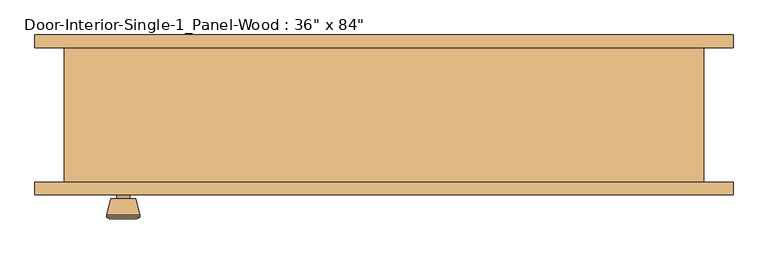
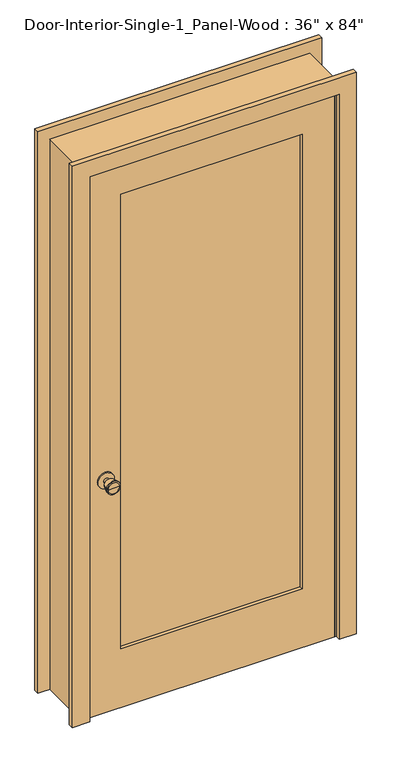
"""IFC4 building model written with IfcOpenShell, lengths in millimetres: door geometry."""

from ifc_helpers import new_model, si_unit, point, frame, frame_2d, origin, place, context, project, spatial, polyline, circle_curve, trimmed, segment, composite_curve, outline, extrude, faceted_brep, source, transform, mapped, element, save
from ifc_brep_helpers import plane_surface, cylinder_surface, revolved_surface, advanced_brep


def door_1a936fe1(model_context):
    return source(origin(), model_context, "Body", "SolidModel", [
        advanced_brep(
        [(-393.7, -57.5, 914.4), (-403.7, -57.5, 914.4), (-383.7, -57.5, 914.4), (-373.2241324, -8.5, 914.4), (-414.1758676, -8.5, 914.4), (-393.7, -8.5, 914.4), (-368.7, -10.3278681, 914.4), (-418.7, -10.3278681, 914.4), (-368.7, -13.7915463, 914.4), (-418.7, -13.7915463, 914.4), (-375.063764, -38.5, 914.4), (-412.336236, -38.5, 914.4), (-383.7, -38.5, 914.4), (-403.7, -38.5, 914.4)],
        [
            (0, 1),
            (1, 2, circle_curve(frame((-393.7, -57.5, 914.4), z_axis=(0.0, -1.0, 0.0), x_axis=(-1.0, 0.0, 0.0)), 10.0)),
            (2, 0),
            (2, 1, circle_curve(frame((-393.7, -57.5, 914.4), z_axis=(0.0, -1.0, 0.0), x_axis=(-1.0, 0.0, 0.0)), 10.0)),
            (3, 4, circle_curve(frame((-393.7, -8.5, 914.4), z_axis=(0.0, 1.0, 0.0), x_axis=(-1.0, 0.0, 0.0)), 20.4758676)),
            (4, 5),
            (5, 3),
            (4, 3, circle_curve(frame((-393.7, -8.5, 914.4), z_axis=(0.0, 1.0, 0.0), x_axis=(-1.0, 0.0, 0.0)), 20.4758676)),
            (6, 7, circle_curve(frame((-393.7, -10.3278681, 914.4), z_axis=(0.0, 1.0, 0.0), x_axis=(-1.0, 0.0, 0.0)), 25.0)),
            (7, 4),
            (3, 6),
            (7, 6, circle_curve(frame((-393.7, -10.3278681, 914.4), z_axis=(0.0, 1.0, 0.0), x_axis=(-1.0, 0.0, 0.0)), 25.0)),
            (8, 9, circle_curve(frame((-393.7, -13.7915463, 914.4), z_axis=(0.0, 1.0, 0.0), x_axis=(-1.0, 0.0, 0.0)), 25.0)),
            (9, 7),
            (6, 8),
            (9, 8, circle_curve(frame((-393.7, -13.7915463, 914.4), z_axis=(0.0, 1.0, 0.0), x_axis=(-1.0, 0.0, 0.0)), 25.0)),
            (10, 11, circle_curve(frame((-393.7, -38.5, 914.4), z_axis=(0.0, 1.0, 0.0), x_axis=(-1.0, 0.0, 0.0)), 18.636236)),
            (11, 9),
            (8, 10),
            (11, 10, circle_curve(frame((-393.7, -38.5, 914.4), z_axis=(0.0, 1.0, 0.0), x_axis=(-1.0, 0.0, 0.0)), 18.636236)),
            (12, 13, circle_curve(frame((-393.7, -38.5, 914.4), z_axis=(0.0, 1.0, 0.0), x_axis=(-1.0, 0.0, 0.0)), 10.0)),
            (13, 11),
            (10, 12),
            (13, 12, circle_curve(frame((-393.7, -38.5, 914.4), z_axis=(0.0, 1.0, 0.0), x_axis=(-1.0, 0.0, 0.0)), 10.0)),
            (1, 13),
            (12, 2),
        ],
        [
            plane_surface(frame((-393.7, -57.5, 914.4), z_axis=(0.0, -1.0, 0.0), x_axis=(-1.0, 0.0, 0.0))),
            plane_surface(frame((-393.7, -8.5, 914.4), z_axis=(0.0, 1.0, 0.0), x_axis=(-1.0, 0.0, 0.0))),
            revolved_surface(polyline([(-414.1758676, -8.5, 914.4), (-418.7, -10.3278681, 914.4)]), (-393.7, -57.5, 914.4), (0.0, -1.0, 0.0)),
            cylinder_surface(frame((-393.7, -57.5, 914.4), z_axis=(0.0, -1.0, 0.0), x_axis=(-1.0, 0.0, 0.0)), 25.0),
            revolved_surface(polyline([(-418.7, -13.7915463, 914.4), (-412.336236, -38.5, 914.4)]), (-393.7, -57.5, 914.4), (0.0, -1.0, 0.0)),
            plane_surface(frame((-393.7, -38.5, 914.4), z_axis=(0.0, -1.0, 0.0), x_axis=(-1.0, 0.0, 0.0))),
            cylinder_surface(frame((-393.7, -57.5, 914.4), z_axis=(0.0, -1.0, 0.0), x_axis=(-1.0, 0.0, 0.0)), 10.0),
        ],
        [
            (0, [[1, 2, 3]]),
            (0, [[-3, 4, -1]]),
            (1, [[5, 6, 7]]),
            (1, [[8, -7, -6]]),
            (2, [[9, 10, -5, 11]]),
            (2, [[12, -11, -8, -10]]),
            (3, [[13, 14, -9, 15]]),
            (3, [[16, -15, -12, -14]]),
            (4, [[17, 18, -13, 19]]),
            (4, [[20, -19, -16, -18]]),
            (5, [[21, 22, -17, 23]]),
            (5, [[24, -23, -20, -22]]),
            (6, [[-2, 25, -21, 26]]),
            (6, [[-4, -26, -24, -25]]),
        ],
    ),
        extrude(outline(composite_curve([segment(trimmed(circle_curve(frame_2d((914.4, -393.7)), 30.0), [point((914.4, -423.7))], [point((914.4, -363.7))], False, "CARTESIAN"), True, "CONTINUOUS"), segment(trimmed(circle_curve(frame_2d((914.4, -393.7)), 30.0), [point((914.4, -363.7))], [point((914.4, -423.7))], False, "CARTESIAN"), True, "CONTINUOUS")], self_intersect=False)), frame((0.0, -63.5, 0.0), z_axis=(0.0, 1.0, 0.0), x_axis=(0.0, 0.0, 1.0)), (0.0, 0.0, 1.0), 6.0),
        advanced_brep(
        [(-393.7, -104.425, 914.4), (-383.7, -104.425, 914.4), (-403.7, -104.425, 914.4), (-373.2241324, -153.425, 914.4), (-393.7, -153.425, 914.4), (-414.1758676, -153.425, 914.4), (-368.7, -151.5971319, 914.4), (-418.7, -151.5971319, 914.4), (-368.7, -148.1334537, 914.4), (-418.7, -148.1334537, 914.4), (-375.063764, -123.425, 914.4), (-412.336236, -123.425, 914.4), (-383.7, -123.425, 914.4), (-403.7, -123.425, 914.4)],
        [
            (0, 1),
            (1, 2, circle_curve(frame((-393.7, -104.425, 914.4), z_axis=(0.0, 1.0, 0.0), x_axis=(-1.0, 0.0, 0.0)), 10.0)),
            (2, 0),
            (2, 1, circle_curve(frame((-393.7, -104.425, 914.4), z_axis=(0.0, 1.0, 0.0), x_axis=(-1.0, 0.0, 0.0)), 10.0)),
            (3, 4),
            (4, 5),
            (5, 3, circle_curve(frame((-393.7, -153.425, 914.4), z_axis=(0.0, -1.0, 0.0), x_axis=(-1.0, 0.0, 0.0)), 20.4758676)),
            (3, 5, circle_curve(frame((-393.7, -153.425, 914.4), z_axis=(0.0, -1.0, 0.0), x_axis=(-1.0, 0.0, 0.0)), 20.4758676)),
            (6, 3),
            (5, 7),
            (7, 6, circle_curve(frame((-393.7, -151.5971319, 914.4), z_axis=(0.0, -1.0, 0.0), x_axis=(-1.0, 0.0, 0.0)), 25.0)),
            (6, 7, circle_curve(frame((-393.7, -151.5971319, 914.4), z_axis=(0.0, -1.0, 0.0), x_axis=(-1.0, 0.0, 0.0)), 25.0)),
            (8, 6),
            (7, 9),
            (9, 8, circle_curve(frame((-393.7, -148.1334537, 914.4), z_axis=(0.0, -1.0, 0.0), x_axis=(-1.0, 0.0, 0.0)), 25.0)),
            (8, 9, circle_curve(frame((-393.7, -148.1334537, 914.4), z_axis=(0.0, -1.0, 0.0), x_axis=(-1.0, 0.0, 0.0)), 25.0)),
            (10, 8),
            (9, 11),
            (11, 10, circle_curve(frame((-393.7, -123.425, 914.4), z_axis=(0.0, -1.0, 0.0), x_axis=(-1.0, 0.0, 0.0)), 18.636236)),
            (10, 11, circle_curve(frame((-393.7, -123.425, 914.4), z_axis=(0.0, -1.0, 0.0), x_axis=(-1.0, 0.0, 0.0)), 18.636236)),
            (12, 10),
            (11, 13),
            (13, 12, circle_curve(frame((-393.7, -123.425, 914.4), z_axis=(0.0, -1.0, 0.0), x_axis=(-1.0, 0.0, 0.0)), 10.0)),
            (12, 13, circle_curve(frame((-393.7, -123.425, 914.4), z_axis=(0.0, -1.0, 0.0), x_axis=(-1.0, 0.0, 0.0)), 10.0)),
            (1, 12),
            (13, 2),
        ],
        [
            plane_surface(frame((-393.7, -104.425, 914.4), z_axis=(0.0, 1.0, 0.0), x_axis=(-1.0, 0.0, 0.0))),
            plane_surface(frame((-393.7, -153.425, 914.4), z_axis=(0.0, -1.0, 0.0), x_axis=(-1.0, 0.0, 0.0))),
            revolved_surface(polyline([(-414.1758676, -153.425, 914.4), (-418.7, -151.5971319, 914.4)]), (-393.7, -104.425, 914.4), (0.0, 1.0, 0.0)),
            cylinder_surface(frame((-393.7, -104.425, 914.4), z_axis=(0.0, 1.0, 0.0), x_axis=(-1.0, 0.0, 0.0)), 25.0),
            revolved_surface(polyline([(-418.7, -148.1334537, 914.4), (-412.336236, -123.425, 914.4)]), (-393.7, -104.425, 914.4), (0.0, 1.0, 0.0)),
            plane_surface(frame((-393.7, -123.425, 914.4), z_axis=(0.0, 1.0, 0.0), x_axis=(-1.0, 0.0, 0.0))),
            cylinder_surface(frame((-393.7, -104.425, 914.4), z_axis=(0.0, 1.0, 0.0), x_axis=(-1.0, 0.0, 0.0)), 10.0),
        ],
        [
            (0, [[1, 2, 3]]),
            (0, [[-3, 4, -1]]),
            (1, [[5, 6, 7]]),
            (1, [[-6, -5, 8]]),
            (2, [[9, -7, 10, 11]]),
            (2, [[-10, -8, -9, 12]]),
            (3, [[13, -11, 14, 15]]),
            (3, [[-14, -12, -13, 16]]),
            (4, [[17, -15, 18, 19]]),
            (4, [[-18, -16, -17, 20]]),
            (5, [[21, -19, 22, 23]]),
            (5, [[-22, -20, -21, 24]]),
            (6, [[25, -23, 26, -2]]),
            (6, [[-26, -24, -25, -4]]),
        ],
    ),
        extrude(outline(composite_curve([segment(trimmed(circle_curve(frame_2d((914.4, -393.7)), 30.0), [point((914.4, -423.7))], [point((914.4, -363.7))], False, "CARTESIAN"), True, "CONTINUOUS"), segment(trimmed(circle_curve(frame_2d((914.4, -393.7)), 30.0), [point((914.4, -363.7))], [point((914.4, -423.7))], False, "CARTESIAN"), True, "CONTINUOUS")], self_intersect=False)), frame((0.0, -104.425, 0.0), z_axis=(0.0, 1.0, 0.0), x_axis=(0.0, 0.0, 1.0)), (0.0, 0.0, 1.0), 6.0),
        faceted_brep([(482.6, -98.425, 0.0), (457.2, -98.425, 0.0), (457.2, -63.5, 0.0), (444.5, -63.5, 0.0), (444.5, -28.575, 0.0), (457.2, -28.575, 0.0), (457.2, 104.775, 0.0), (482.6, 104.775, 0.0), (482.6, 104.775, 2159.0), (482.6, -98.425, 2159.0), (457.2, 104.775, 2133.6), (-457.2, 104.775, 2133.6), (-457.2, 104.775, 0.0), (-482.6, 104.775, 0.0), (-482.6, 104.775, 2159.0), (457.2, -28.575, 2133.6), (444.5, -28.575, 2120.9), (-444.5, -28.575, 2120.9), (-444.5, -28.575, 0.0), (-457.2, -28.575, 0.0), (-457.2, -28.575, 2133.6), (444.5, -63.5, 2120.9), (457.2, -63.5, 2133.6), (-457.2, -63.5, 2133.6), (-457.2, -63.5, 0.0), (-444.5, -63.5, 0.0), (-444.5, -63.5, 2120.9), (457.2, -98.425, 2133.6), (-482.6, -98.425, 2159.0), (-482.6, -98.425, 0.0), (-457.2, -98.425, 0.0), (-457.2, -98.425, 2133.6)], [[[0, 1, 2, 3, 4, 5, 6, 7]], [[7, 8, 9, 0]], [[6, 10, 11, 12, 13, 14, 8, 7]], [[5, 15, 10, 6]], [[4, 16, 17, 18, 19, 20, 15, 5]], [[3, 21, 16, 4]], [[2, 22, 23, 24, 25, 26, 21, 3]], [[1, 27, 22, 2]], [[0, 9, 28, 29, 30, 31, 27, 1]], [[8, 14, 28, 9]], [[15, 20, 11, 10]], [[21, 26, 17, 16]], [[27, 31, 23, 22]], [[29, 13, 12, 19, 18, 25, 24, 30]], [[14, 13, 29, 28]], [[20, 19, 12, 11]], [[26, 25, 18, 17]], [[31, 30, 24, 23]]]),
        extrude(outline(polyline([(2133.6, -457.2), (0.0, -457.2), (0.0, 457.2), (2133.6, 457.2), (2133.6, -457.2)]), holes=[polyline([(2014.5375, -336.55), (2014.5375, 336.55), (231.775, 336.55), (231.775, -336.55), (2014.5375, -336.55)])]), frame((0.0, -98.425, 0.0), z_axis=(0.0, 1.0, 0.0), x_axis=(0.0, 0.0, 1.0)), (0.0, 0.0, 1.0), 34.925),
        extrude(outline(polyline([(336.55, -75.1416667), (336.55, -86.7833333), (-336.55, -86.7833333), (-336.55, -75.1416667), (336.55, -75.1416667)])), frame((0.0, 0.0, 231.775), z_axis=(0.0, 0.0, 1.0), x_axis=(1.0, 0.0, 0.0)), (0.0, 0.0, 1.0), 1782.7625),
        extrude(outline(polyline([(0.0, 527.05), (2203.45, 527.05), (2203.45, -527.05), (0.0, -527.05), (0.0, -463.55), (2139.95, -463.55), (2139.95, 463.55), (0.0, 463.55), (0.0, 527.05)])), frame((0.0, -117.475, 0.0), z_axis=(0.0, 1.0, 0.0), x_axis=(0.0, 0.0, 1.0)), (0.0, 0.0, 1.0), 19.05),
        extrude(outline(polyline([(0.0, 527.05), (2203.45, 527.05), (2203.45, -527.05), (0.0, -527.05), (0.0, -463.55), (2139.95, -463.55), (2139.95, 463.55), (0.0, 463.55), (0.0, 527.05)])), frame((0.0, 104.775, 0.0), z_axis=(0.0, 1.0, 0.0), x_axis=(0.0, 0.0, 1.0)), (0.0, 0.0, 1.0), 19.05),
    ])


if __name__ == "__main__":
    model = new_model("IFC4")
    model_context = context("Model", 3, world=origin())
    ifc_project = project(units=[si_unit("LENGTHUNIT", "METRE", prefix="MILLI")], contexts=[model_context])
    site = spatial("IfcSite", under=ifc_project)
    building = spatial("IfcBuilding", under=site)
    placement = place(None, origin())
    door_shape = door_1a936fe1(model_context)
    element("IfcDoor", 1, ObjectType="Door-Interior-Single-1_Panel-Wood : 36\" x 84\"", at=placement, inside=building, context=model_context, shape_type="MappedRepresentation", body=[
        mapped(door_shape, transform((0.0, 0.0, 0.0), x_axis=(1.0, 0.0, 0.0), y_axis=(0.0, 1.0, 0.0), z_axis=(0.0, 0.0, 1.0))),
    ])
    save(model, "model.ifc")

# Revit data of these elements
# Type "Door-Interior-Single-1_Panel-Wood : 36\" x 84\""
#   Type Mark = "10"
#   Analytic Construction = "Wooden"
#   Top Rail = 0' - 4 11/16"
#   Thickness = 0' - 1 3/8"
#   Thermal Resistance (R) = 2.5876 (h·ft²·°F)/BTU
#   Swing Angle [instance default] = 90.00°
#   Stiles = 0' - 4 3/4"
#   Rough Width = 3' - 2"
#   Rough Height = 7' - 1"
#   Height = 7' - 0"
#   Width = 3' - 0"
#   Heat Transfer Coefficient (U) = 0.3865 BTU/(h·ft²·°F)
#   Bottom Rail = 0' - 9 1/8"
#   Trim Material = Cherry
#   Panel Material = Cherry
#   Frame Material = Cherry
#   Door Handle Material = Aluminum
#   Visual Light Transmittance = 0
#   Solar Heat Gain Coefficient = 0
#   Wall Closure = (empty or 0)
#   Function = (empty or 0)
# Element 1 (IfcDoor, "Door-Interior-Single-1_Panel-Wood : 36\" x 84\"")
#   Materials on its faces: "Cherry", "Aluminum"
# Materials
#   "Cherry": class "Wood", colour RGB 226 177 128, transparency 0, Description = "Prunus Serotina", Cost = 0
#   "Aluminum": class "Metal", colour RGB 247 247 247, transparency 0, Description = "Aluminum 6061", Cost = 0
